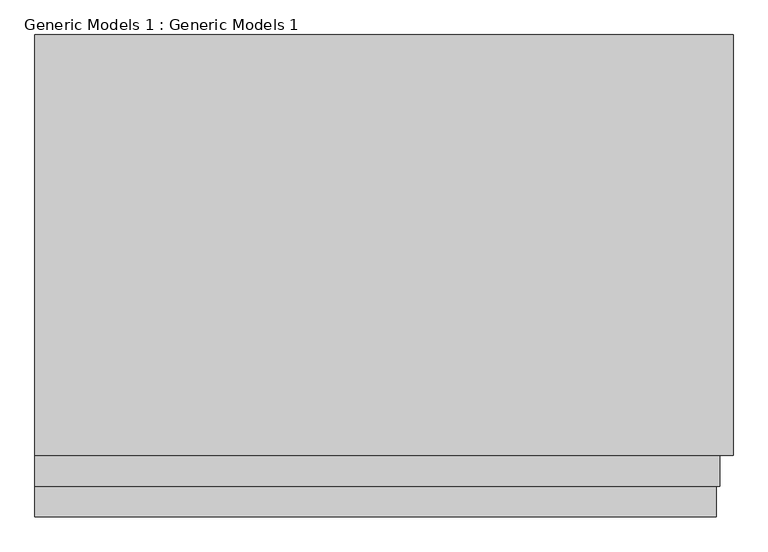
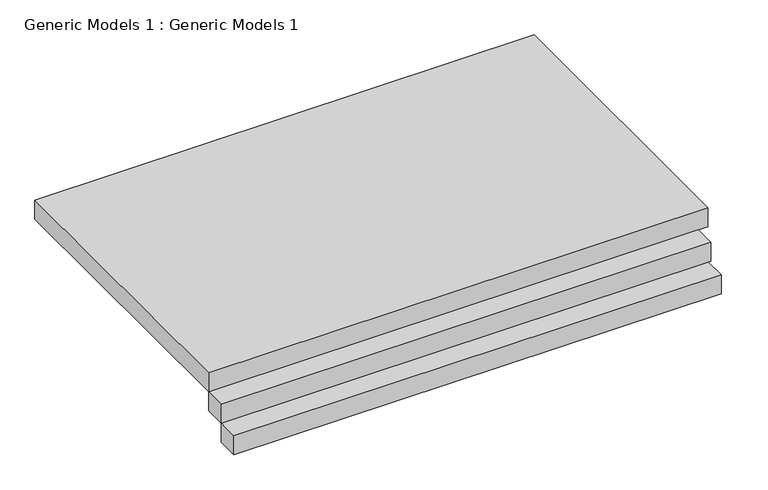
"""IFC4 building model written with IfcOpenShell, lengths in millimetres: proxy geometry, Generic Models 1 : Generic Models 1."""

from ifc_helpers import new_model, si_unit, frame, origin, origin_with_axes, place, context, project, spatial, polyline, outline, extrude, source, transform, mapped, element, save


def generic_models_1_generic_models_1_d0396bf3(model_context):
    return source(origin(), model_context, "Body", "SweptSolid", [
        extrude(outline(polyline([(-7860.2229687, -11454.2125482), (-7860.2229687, -11124.0125482), (-462.6995143, -11124.0125482), (-462.6995143, -11454.2125482), (-7860.2229687, -11454.2125482)])), frame((0.0, 0.0, -609.6), z_axis=(0.0, 0.0, 1.0), x_axis=(1.0, 0.0, 0.0)), (0.0, 0.0, 1.0), 304.8),
        extrude(outline(polyline([(-425.5154257, -10789.7015118), (-425.5154257, -11124.0125482), (-7860.2229687, -11124.0125482), (-7860.2229687, -10789.7015118), (-425.5154257, -10789.7015118)])), frame((0.0, 0.0, -304.8), z_axis=(0.0, 0.0, 1.0), x_axis=(1.0, 0.0, 0.0)), (0.0, 0.0, 1.0), 304.8),
        extrude(outline(polyline([(-279.2605133, -6217.7015118), (-279.2605133, -10789.7015118), (-7860.2229687, -10789.7015118), (-7860.2229687, -6217.7015118), (-279.2605133, -6217.7015118)])), origin_with_axes(), (0.0, 0.0, 1.0), 304.8),
    ])


if __name__ == "__main__":
    model = new_model("IFC4")
    model_context = context("Model", 3, world=origin())
    ifc_project = project(units=[si_unit("LENGTHUNIT", "METRE", prefix="MILLI")], contexts=[model_context])
    site = spatial("IfcSite", under=ifc_project)
    building = spatial("IfcBuilding", under=site)
    placement = place(None, origin())
    generic_models_1_generic_models_1_shape = generic_models_1_generic_models_1_d0396bf3(model_context)
    element("IfcBuildingElementProxy", 1, Name="Generic Models 1 : Generic Models 1", ObjectType="Generic Models 1 : Generic Models 1", at=placement, inside=building, context=model_context, shape_type="MappedRepresentation", body=[
        mapped(generic_models_1_generic_models_1_shape, transform((0.0, 0.0, 0.0), x_axis=(1.0, 0.0, 0.0), y_axis=(0.0, 1.0, 0.0), z_axis=(0.0, 0.0, 1.0))),
    ])
    save(model, "model.ifc")
